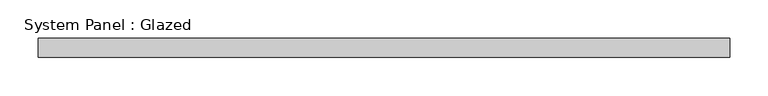
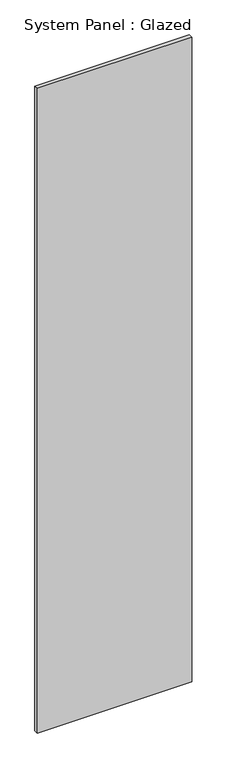
"""IFC4 building model written with IfcOpenShell, lengths in millimetres: plate geometry, System Panel : Glazed."""

from ifc_helpers import new_model, si_unit, origin, origin_with_axes, place, context, project, spatial, polyline, outline, extrude, source, transform, mapped, element, save


def system_panel_glazed_1225bd09(model_context):
    return source(origin(), model_context, "Body", "SweptSolid", [
        extrude(outline(polyline([(453.1301593, 24.5), (-453.1301593, 24.5), (-453.1301593, 49.5), (453.1301593, 49.5), (453.1301593, 24.5)])), origin_with_axes(), (0.0, 0.0, 1.0), 4000.0),
    ])


if __name__ == "__main__":
    model = new_model("IFC4")
    model_context = context("Model", 3, world=origin())
    ifc_project = project(units=[si_unit("LENGTHUNIT", "METRE", prefix="MILLI")], contexts=[model_context])
    site = spatial("IfcSite", under=ifc_project)
    building = spatial("IfcBuilding", under=site)
    placement = place(None, origin())
    system_panel_glazed_shape = system_panel_glazed_1225bd09(model_context)
    element("IfcPlate", 1, ObjectType="System Panel : Glazed", at=placement, inside=building, context=model_context, shape_type="MappedRepresentation", body=[
        mapped(system_panel_glazed_shape, transform((0.0, 0.0, 0.0), x_axis=(1.0, 0.0, 0.0), y_axis=(0.0, 1.0, 0.0), z_axis=(0.0, 0.0, 1.0))),
    ])
    save(model, "model.ifc")

# Revit data of these elements
# Type "System Panel : Glazed"
#   Keynote = "H11"
#   Construction Type Id = "GSP4R"
#   Analytic Construction = "1/8 in Pilkington single glazing"
#   Visual Light Transmittance = 0.9
#   Solar Heat Gain Coefficient = 0.86
#   Heat Transfer Coefficient (U) = 6.7069 W/(m²·K)
#   Define Thermal Properties by = 1
# Element 1 (IfcPlate, "System Panel : Glazed")
#   Materials on its faces: "Glass"
# Materials
#   "Glass": class "Glass", colour RGB 0 128 192, transparency 0.9, Description = "Soda Lime Glass", Cost = 0
